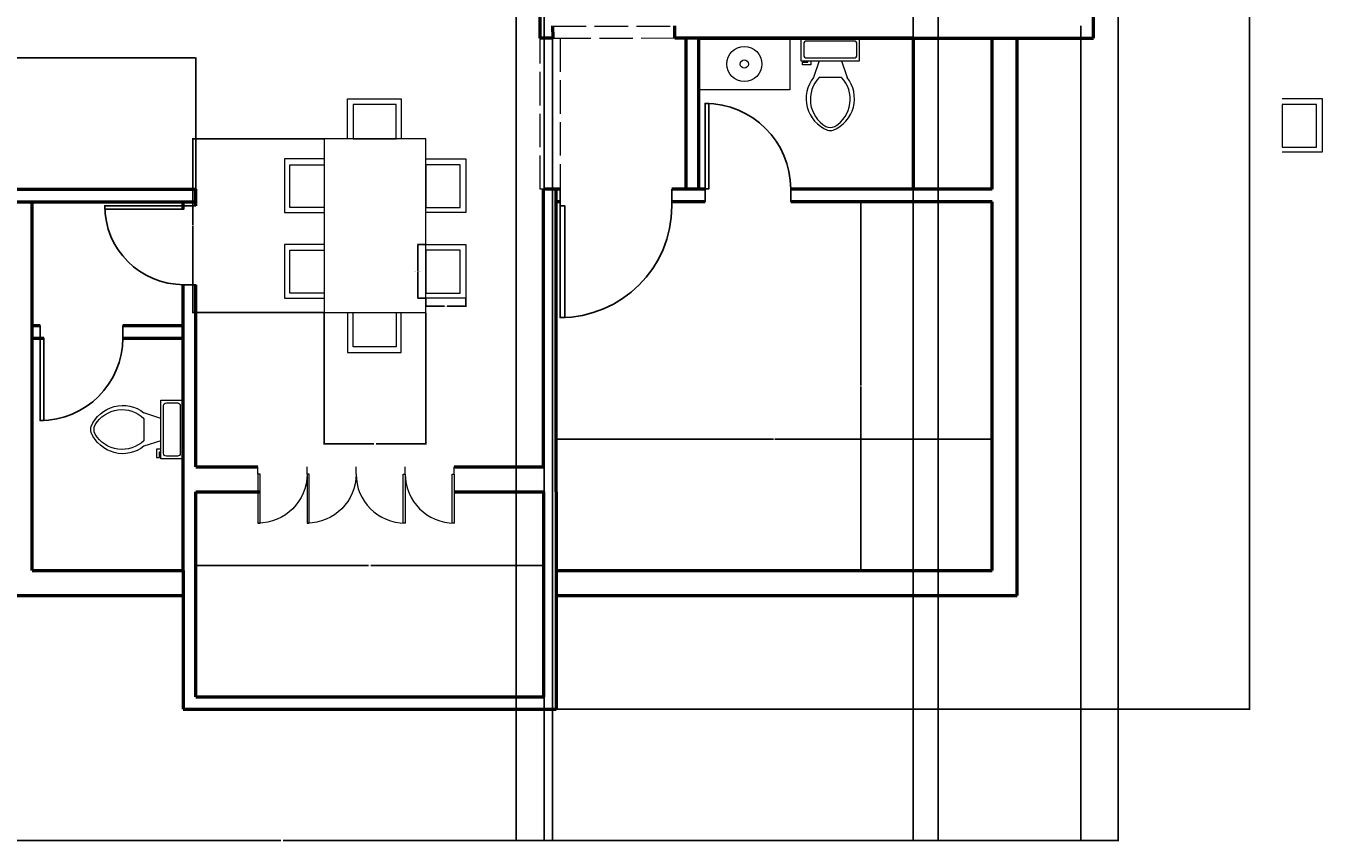
# Model space of a CAD drawing. Units: inches. Extents: x 2032 to 3981, y 840 to 2177.
# Tile 2 of 6: x 2286 to 2750, y 840 to 1132. Entities that reach past the tile are written whole.
import ezdxf

# ---------------------------------------------------------------- set-up
doc = ezdxf.new("R2010")
doc.units = ezdxf.units.IN
doc.linetypes.add('ACAD_ISO02W100', pattern=[15, 12, -3])
for name, color, linetype, lineweight in [('A-ANNO-DIMS', 2, 'Continuous', 18), ('A-DOOR', 3, 'Continuous', 25), ('A-FLOR-FIXT', 9, 'Continuous', 18), ('A-FURN', 8, 'Continuous', 18), ('A-GLAZ', 4, 'Continuous', 18), ('A-WALL', 7, 'Continuous', 50), ('A-WALL-OVHD', 8, 'ACAD_ISO02W100', 18)]:
    doc.layers.add(name, color=color, linetype=linetype, lineweight=lineweight)
doc.styles.get("Standard").update_dxf_attribs({"font": 'arial.ttf'})
doc.dimstyles.get("Standard").update_dxf_attribs({"dimtxt": 0.18, "dimasz": 0.18, "dimexe": 0.18, "dimexo": 0.0625, "dimgap": 0.09, "dimtad": 0, "dimtih": 1, "dimtoh": 1, "dimdec": 4, "dimzin": 0, "dimdsep": 46, "dimtxsty": 'Standard', "dimcen": 0.09, "dimadec": 0, "dimazin": 0, "dimtfac": 1, "dimtdec": 4, "dimtofl": 0, "dimtmove": 0, "dimatfit": 3, "dimfxl": 1, "dimtolj": 1, "dimtzin": 0, "dimarcsym": 0})

# ---------------------------------------------------------------- blocks, each defined once
blk = doc.blocks.new('*U2')
for p, q in [((0, 0), (0, -6)), ((40, 0), (40, -6))]:
    blk.add_line(p, q)
blk.add_lwpolyline([(0, 0), (0, 40), (1.75, 40), (1.75, 0)], close=True)
blk.add_arc((0, 0), 40, 0, 90)
blk = doc.blocks.new('*U4')
for p, q in [((9.5, -6), (9.5, -2)), ((-10, -8.5), (-8, -8.5)), ((-10, -9.5), (-10, -8.5)), ((-8, -8.5), (-8, -8)), ((-7, -8), (-7, -9.5)), ((-4, -8), (-6, -14)), ((4, -8), (6, -14)), ((-7, -9.5), (-10, -9.5)), ((4, -14), (-4, -14))]:
    blk.add_line(p, q)
blk.add_lwpolyline([(10.5, -8), (10.5, 0), (-10.5, 0), (-10.5, -8)], close=True)
for points in [[(-9.5, -2), (-9.5, -6)], [(8.5, -1), (-8.5, -1)], [(-8.5, -7), (8.5, -7)]]:
    blk.add_lwpolyline(points)
for centre, radius, start, end in [((-8.62, -1.88), 0.884, 81.8699, 188.1301), ((8.62, -1.88), 0.884, 351.8699, 98.1301), ((-8.62, -6.12), 0.884, 171.8699, 278.1301), ((8.62, -6.12), 0.884, 261.8699, 8.1301), ((3.52, -21.58), 12.17, 141.4691, 247.9714), ((4.2, -21.82), 11.33, 136.3677, 238.9468), ((-3.52, -21.58), 12.17, 292.0284, 38.5307), ((-4.2, -21.82), 11.33, 301.053, 43.6321), ((0, -27.88), 4, 245.7318, 294.2682), ((0, -29), 4, 254.8605, 285.1395)]:
    blk.add_arc(centre, radius, start, end)
blk = doc.blocks.new('CHAIR-DINING')
for p, q in [((0, 0), (0, 14.22)), ((0, 14.22), (19.23, 14.22)), ((19.23, 14.22), (19.23, 0))]:
    blk.add_line(p, q)
blk.add_lwpolyline([(2.09, 0), (17.42, 0), (17.42, 12.28), (2.09, 12.28)], close=True)
blk = doc.blocks.new('*D8')
at = {"layer": 'A-ANNO-DIMS', "color": 0, "lineweight": -2, "transparency": 16777216}
for p, q in [((2429.55, 1053.69), (2426.55, 1053.69)), ((2426.73, 1053.51), (2426.73, 1044.26)), ((2426.73, 1034.64), (2426.73, 1043.89)), ((2429.55, 1034.46), (2426.55, 1034.46))]:
    blk.add_line(p, q, dxfattribs=at)
at = {"layer": 'A-ANNO-DIMS', "color": 0, "lineweight": 100, "transparency": 16777216}
for points in [[(2426.7, 1053.51), (2426.76, 1053.51), (2426.73, 1053.69)], [(2426.7, 1034.64), (2426.76, 1034.64), (2426.73, 1034.46)]]:
    blk.add_solid(points, dxfattribs=at)
at = {"layer": 'Defpoints', "color": 0, "lineweight": 100, "transparency": 16777216}
for p in [(2429.61, 1053.69), (2426.73, 1034.46), (2429.61, 1034.46)]:
    blk.add_point(p, dxfattribs=at)
at = {"layer": 'A-ANNO-DIMS', "color": 0, "transparency": 16777216, "insert": (2426.73, 1044.07), "char_height": 0.18, "attachment_point": 5}
blk.add_mtext('\\A1;DINING CHAIR 19 TYP.', dxfattribs=at)
blk = doc.blocks.new('*D9')
at = {"layer": 'A-ANNO-DIMS', "color": 0, "lineweight": -2, "transparency": 16777216}
for p, q in [((2429.61, 1034.4), (2429.61, 1031.39)), ((2443.83, 1034.4), (2443.83, 1031.39)), ((2429.79, 1031.57), (2436.2, 1031.57)), ((2443.65, 1031.57), (2437.24, 1031.57))]:
    blk.add_line(p, q, dxfattribs=at)
at = {"layer": 'A-ANNO-DIMS', "color": 0, "lineweight": 100, "transparency": 16777216}
for points in [[(2429.79, 1031.6), (2429.79, 1031.54), (2429.61, 1031.57)], [(2443.65, 1031.6), (2443.65, 1031.54), (2443.83, 1031.57)]]:
    blk.add_solid(points, dxfattribs=at)
at = {"layer": 'Defpoints', "color": 0, "lineweight": 100, "transparency": 16777216}
for p in [(2429.61, 1034.46), (2443.83, 1034.46), (2443.83, 1031.57)]:
    blk.add_point(p, dxfattribs=at)
at = {"layer": 'A-ANNO-DIMS', "color": 0, "transparency": 16777216, "insert": (2436.72, 1031.57), "char_height": 0.18, "attachment_point": 5}
blk.add_mtext('\\A1;14 TYP.', dxfattribs=at)
blk = doc.blocks.new('*D14')
at = {"layer": 'A-ANNO-DIMS', "color": 0, "lineweight": -2, "transparency": 16777216}
for p, q in [((2078.89, 1518.9), (2078.89, 840.08)), ((2677.35, 1476.9), (2677.35, 840.08)), ((2079.07, 840.26), (2377.73, 840.26)), ((2677.17, 840.26), (2378.52, 840.26))]:
    blk.add_line(p, q, dxfattribs=at)
at = {"layer": 'A-ANNO-DIMS', "color": 0, "lineweight": 100, "transparency": 16777216}
for points in [[(2079.07, 840.29), (2079.07, 840.23), (2078.89, 840.26)], [(2677.17, 840.29), (2677.17, 840.23), (2677.35, 840.26)]]:
    blk.add_solid(points, dxfattribs=at)
at = {"layer": 'Defpoints', "color": 0, "lineweight": 100, "transparency": 16777216}
for p in [(2078.89, 1518.96), (2677.35, 1476.96), (2677.35, 840.26)]:
    blk.add_point(p, dxfattribs=at)
at = {"layer": 'A-ANNO-DIMS', "color": 0, "transparency": 16777216, "insert": (2378.12, 840.26), "char_height": 0.18, "attachment_point": 5}
blk.add_mtext('\\A1;598.5', dxfattribs=at)
blk = doc.blocks.new('*D15')
at = {"layer": 'A-ANNO-DIMS', "color": 0, "lineweight": -2, "transparency": 16777216}
for p, q in [((2456.69, 1820.52), (2724.53, 1820.52)), ((2724.35, 1820.34), (2724.35, 1354.07)), ((2724.35, 887.44), (2724.35, 1353.71)), ((2476.27, 887.26), (2724.53, 887.26))]:
    blk.add_line(p, q, dxfattribs=at)
at = {"layer": 'A-ANNO-DIMS', "color": 0, "lineweight": 100, "transparency": 16777216}
for points in [[(2724.32, 1820.34), (2724.38, 1820.34), (2724.35, 1820.52)], [(2724.32, 887.44), (2724.38, 887.44), (2724.35, 887.26)]]:
    blk.add_solid(points, dxfattribs=at)
at = {"layer": 'Defpoints', "color": 0, "lineweight": 100, "transparency": 16777216}
for p in [(2456.63, 1820.52), (2476.21, 887.26), (2724.35, 887.26)]:
    blk.add_point(p, dxfattribs=at)
at = {"layer": 'A-ANNO-DIMS', "color": 0, "transparency": 16777216, "insert": (2724.35, 1353.89), "char_height": 0.18, "attachment_point": 5}
blk.add_mtext('\\A1;933.3', dxfattribs=at)
blk = doc.blocks.new('*D44')
at = {"layer": 'A-ANNO-DIMS', "color": 0, "lineweight": -2, "transparency": 16777216}
for p, q in [((2164.21, 1073.52), (2164.21, 1120.64)), ((2164.39, 1120.46), (2255.43, 1120.46)), ((2347.03, 1120.46), (2255.99, 1120.46)), ((2347.21, 1073.52), (2347.21, 1120.64))]:
    blk.add_line(p, q, dxfattribs=at)
at = {"layer": 'A-ANNO-DIMS', "color": 0, "lineweight": 100, "transparency": 16777216}
for points in [[(2164.39, 1120.49), (2164.39, 1120.43), (2164.21, 1120.46)], [(2347.03, 1120.49), (2347.03, 1120.43), (2347.21, 1120.46)]]:
    blk.add_solid(points, dxfattribs=at)
at = {"layer": 'Defpoints', "color": 0, "lineweight": 100, "transparency": 16777216}
for p in [(2347.21, 1120.46), (2164.21, 1073.46), (2347.21, 1073.46)]:
    blk.add_point(p, dxfattribs=at)
at = {"layer": 'A-ANNO-DIMS', "color": 0, "transparency": 16777216, "insert": (2255.71, 1120.46), "char_height": 0.18, "attachment_point": 5}
blk.add_mtext('\\A1;183', dxfattribs=at)
blk = doc.blocks.new('*D46')
at = {"layer": 'A-ANNO-DIMS', "color": 0, "lineweight": -2, "transparency": 16777216}
for p, q in [((2347.21, 891.82), (2347.21, 938.94)), ((2347.39, 938.76), (2409.07, 938.76)), ((2471.53, 938.76), (2409.85, 938.76)), ((2471.71, 891.82), (2471.71, 938.94))]:
    blk.add_line(p, q, dxfattribs=at)
at = {"layer": 'A-ANNO-DIMS', "color": 0, "lineweight": 100, "transparency": 16777216}
for points in [[(2347.39, 938.79), (2347.39, 938.73), (2347.21, 938.76)], [(2471.53, 938.79), (2471.53, 938.73), (2471.71, 938.76)]]:
    blk.add_solid(points, dxfattribs=at)
at = {"layer": 'Defpoints', "color": 0, "lineweight": 100, "transparency": 16777216}
for p in [(2471.71, 938.76), (2347.21, 891.76), (2471.71, 891.76)]:
    blk.add_point(p, dxfattribs=at)
at = {"layer": 'A-ANNO-DIMS', "color": 0, "transparency": 16777216, "insert": (2409.46, 938.76), "char_height": 0.18, "attachment_point": 5}
blk.add_mtext('\\A1;124.5', dxfattribs=at)
blk = doc.blocks.new('*D47')
at = {"layer": 'A-ANNO-DIMS', "color": 0, "lineweight": -2, "transparency": 16777216}
for p, q in [((2476.21, 937.02), (2476.21, 984.14)), ((2476.39, 983.96), (2553.93, 983.96)), ((2632.03, 983.96), (2554.49, 983.96)), ((2632.21, 937.02), (2632.21, 984.14))]:
    blk.add_line(p, q, dxfattribs=at)
at = {"layer": 'A-ANNO-DIMS', "color": 0, "lineweight": 100, "transparency": 16777216}
for points in [[(2476.39, 983.99), (2476.39, 983.93), (2476.21, 983.96)], [(2632.03, 983.99), (2632.03, 983.93), (2632.21, 983.96)]]:
    blk.add_solid(points, dxfattribs=at)
at = {"layer": 'Defpoints', "color": 0, "lineweight": 100, "transparency": 16777216}
for p in [(2632.21, 983.96), (2476.21, 936.96), (2632.21, 936.96)]:
    blk.add_point(p, dxfattribs=at)
at = {"layer": 'A-ANNO-DIMS', "color": 0, "transparency": 16777216, "insert": (2554.21, 983.96), "char_height": 0.18, "attachment_point": 5}
blk.add_mtext('\\A1;156', dxfattribs=at)
blk = doc.blocks.new('*D48')
at = {"layer": 'A-ANNO-DIMS', "color": 0, "lineweight": -2, "transparency": 16777216}
for p, q in [((2632.15, 1068.96), (2585.03, 1068.96)), ((2585.21, 1068.78), (2585.21, 1003.14)), ((2585.21, 937.14), (2585.21, 1002.78)), ((2632.15, 936.96), (2585.03, 936.96))]:
    blk.add_line(p, q, dxfattribs=at)
at = {"layer": 'A-ANNO-DIMS', "color": 0, "lineweight": 100, "transparency": 16777216}
for points in [[(2585.18, 1068.78), (2585.24, 1068.78), (2585.21, 1068.96)], [(2585.18, 937.14), (2585.24, 937.14), (2585.21, 936.96)]]:
    blk.add_solid(points, dxfattribs=at)
at = {"layer": 'Defpoints', "color": 0, "lineweight": 100, "transparency": 16777216}
for p in [(2585.21, 1068.96), (2632.21, 1068.96), (2632.21, 936.96)]:
    blk.add_point(p, dxfattribs=at)
at = {"layer": 'A-ANNO-DIMS', "color": 0, "transparency": 16777216, "insert": (2585.21, 1002.96), "char_height": 0.18, "attachment_point": 5}
blk.add_mtext('\\A1;132', dxfattribs=at)
blk = doc.blocks.new('*D49')
at = {"layer": 'A-ANNO-DIMS', "color": 0, "lineweight": -2, "transparency": 16777216}
for p, q in [((2393.15, 1029.19), (2393.15, 982.07)), ((2429.61, 1029.19), (2429.61, 982.07)), ((2393.33, 982.25), (2410.99, 982.25)), ((2429.43, 982.25), (2411.77, 982.25))]:
    blk.add_line(p, q, dxfattribs=at)
at = {"layer": 'A-ANNO-DIMS', "color": 0, "lineweight": 100, "transparency": 16777216}
for points in [[(2393.33, 982.28), (2393.33, 982.22), (2393.15, 982.25)], [(2429.43, 982.28), (2429.43, 982.22), (2429.61, 982.25)]]:
    blk.add_solid(points, dxfattribs=at)
at = {"layer": 'Defpoints', "color": 0, "lineweight": 100, "transparency": 16777216}
for p in [(2393.15, 1029.25), (2429.61, 1029.25), (2393.15, 982.25)]:
    blk.add_point(p, dxfattribs=at)
at = {"layer": 'A-ANNO-DIMS', "color": 0, "transparency": 16777216, "insert": (2411.38, 982.25), "char_height": 0.18, "attachment_point": 5}
blk.add_mtext('\\A1;36.46', dxfattribs=at)
blk = doc.blocks.new('*D50')
at = {"layer": 'A-ANNO-DIMS', "color": 0, "lineweight": -2, "transparency": 16777216}
for p, q in [((2393.09, 1091.52), (2345.97, 1091.52)), ((2346.15, 1091.34), (2346.15, 1060.57)), ((2346.15, 1029.43), (2346.15, 1060.2)), ((2393.09, 1029.25), (2345.97, 1029.25))]:
    blk.add_line(p, q, dxfattribs=at)
at = {"layer": 'A-ANNO-DIMS', "color": 0, "lineweight": 100, "transparency": 16777216}
for points in [[(2346.12, 1091.34), (2346.18, 1091.34), (2346.15, 1091.52)], [(2346.12, 1029.43), (2346.18, 1029.43), (2346.15, 1029.25)]]:
    blk.add_solid(points, dxfattribs=at)
at = {"layer": 'Defpoints', "color": 0, "lineweight": 100, "transparency": 16777216}
for p in [(2346.15, 1091.52), (2393.15, 1091.52), (2393.15, 1029.25)]:
    blk.add_point(p, dxfattribs=at)
at = {"layer": 'A-ANNO-DIMS', "color": 0, "transparency": 16777216, "insert": (2346.15, 1060.39), "char_height": 0.18, "attachment_point": 5}
blk.add_mtext('\\A1;62.27', dxfattribs=at)
blk = doc.blocks.new('*D56')
at = {"layer": 'A-ANNO-DIMS', "color": 0, "lineweight": -2, "transparency": 16777216}
for p, q in [((2603.93, 1136.83), (2603.93, 840.08)), ((2474.93, 1131.9), (2474.93, 840.08)), ((2475.11, 840.26), (2539.15, 840.26)), ((2603.75, 840.26), (2539.72, 840.26))]:
    blk.add_line(p, q, dxfattribs=at)
at = {"layer": 'A-ANNO-DIMS', "color": 0, "lineweight": 100, "transparency": 16777216}
for points in [[(2475.11, 840.29), (2475.11, 840.23), (2474.93, 840.26)], [(2603.75, 840.29), (2603.75, 840.23), (2603.93, 840.26)]]:
    blk.add_solid(points, dxfattribs=at)
at = {"layer": 'Defpoints', "color": 0, "lineweight": 100, "transparency": 16777216}
for p in [(2603.93, 1136.9), (2474.93, 1131.96), (2603.93, 840.26)]:
    blk.add_point(p, dxfattribs=at)
at = {"layer": 'A-ANNO-DIMS', "color": 0, "transparency": 16777216, "insert": (2539.43, 840.26), "char_height": 0.18, "attachment_point": 5}
blk.add_mtext('\\A1;129', dxfattribs=at)
blk = doc.blocks.new('*D57')
at = {"layer": 'A-ANNO-DIMS', "color": 0, "lineweight": -2, "transparency": 16777216}
for p, q in [((2612.93, 1138.58), (2612.93, 840.08)), ((2663.93, 1131.9), (2663.93, 840.08)), ((2613.11, 840.26), (2638.23, 840.26)), ((2663.75, 840.26), (2638.64, 840.26))]:
    blk.add_line(p, q, dxfattribs=at)
at = {"layer": 'A-ANNO-DIMS', "color": 0, "lineweight": 100, "transparency": 16777216}
for points in [[(2613.11, 840.29), (2613.11, 840.23), (2612.93, 840.26)], [(2663.75, 840.29), (2663.75, 840.23), (2663.93, 840.26)]]:
    blk.add_solid(points, dxfattribs=at)
at = {"layer": 'Defpoints', "color": 0, "lineweight": 100, "transparency": 16777216}
for p in [(2612.93, 1138.65), (2663.93, 1131.96), (2663.93, 840.26)]:
    blk.add_point(p, dxfattribs=at)
at = {"layer": 'A-ANNO-DIMS', "color": 0, "transparency": 16777216, "insert": (2638.43, 840.26), "char_height": 0.18, "attachment_point": 5}
blk.add_mtext('\\A1;51', dxfattribs=at)
blk = doc.blocks.new('*D65')
at = {"layer": 'A-ANNO-DIMS', "color": 0, "lineweight": -2, "transparency": 16777216}
for p, q in [((2461.93, 1358.4), (2461.93, 840.08)), ((2471.93, 1358.4), (2471.93, 840.08)), ((2462.11, 840.26), (2466.72, 840.26)), ((2471.75, 840.26), (2467.14, 840.26))]:
    blk.add_line(p, q, dxfattribs=at)
at = {"layer": 'A-ANNO-DIMS', "color": 0, "lineweight": 100, "transparency": 16777216}
for points in [[(2462.11, 840.29), (2462.11, 840.23), (2461.93, 840.26)], [(2471.75, 840.29), (2471.75, 840.23), (2471.93, 840.26)]]:
    blk.add_solid(points, dxfattribs=at)
at = {"layer": 'Defpoints', "color": 0, "lineweight": 100, "transparency": 16777216}
for p in [(2461.93, 1358.46), (2471.93, 1358.46), (2471.93, 840.26)]:
    blk.add_point(p, dxfattribs=at)
at = {"layer": 'A-ANNO-DIMS', "color": 0, "transparency": 16777216, "insert": (2466.93, 840.26), "char_height": 0.18, "attachment_point": 5}
blk.add_mtext('\\A1;10', dxfattribs=at)

msp = doc.modelspace()

# ---------------------------------------------------------------- linework, layer by layer
at = {"layer": 'A-FLOR-FIXT'}
msp.add_lwpolyline([(2527.2092, 1127.4584), (2559.8471, 1127.4584), (2559.8471, 1109.0275), (2527.2092, 1109.0275)], close=True, dxfattribs=at)
for radius in [6.2897, 1.4782]:
    msp.add_circle((2543.5282, 1118.2429), radius, dxfattribs=at)
at = {"layer": 'A-FURN'}
msp.add_lwpolyline([(2393.15, 1029.2517), (2429.61, 1029.2517), (2429.61, 1091.5219), (2393.15, 1091.5219)], close=True, dxfattribs=at)
at = {"layer": 'A-WALL'}
for p, q in [((2668.4346, 1127.4584), (2668.4346, 1239.9584)), ((2470.4346, 1127.4584), (2470.4346, 1230.9584)), ((2474.9346, 1131.9584), (2475.0017, 1127.4584)), ((2518.6525, 1127.4584), (2518.6525, 1131.9584)), ((2475.0017, 1127.4584), (2470.4346, 1127.4584)), ((2475.0017, 1127.4584), (2475.0017, 1127.4584)), ((2603.9346, 1127.4584), (2518.6525, 1127.4584)), ((2522.7092, 1073.4584), (2522.7092, 1127.4584)), ((2527.2092, 1073.4584), (2527.2092, 1127.4584)), ((2527.2092, 1127.4584), (2668.4346, 1127.4584)), ((2603.9346, 1127.4584), (2603.9346, 1073.4584)), ((2632.2092, 1073.4584), (2632.2092, 1127.4584)), ((2641.2092, 1073.4584), (2641.2092, 1127.4584)), ((2164.2092, 1073.4584), (2347.2092, 1073.4584)), ((2347.2092, 1067.5396), (2347.2092, 1073.4584)), ((2471.7092, 974.088), (2471.7092, 1073.4584)), ((2477.5882, 1073.4584), (2471.7092, 1073.4584)), ((2476.2092, 965.088), (2476.2092, 1073.4584)), ((2529.4826, 1073.4584), (2517.5882, 1073.4584)), ((2529.4826, 1073.4584), (2527.2092, 1073.4584)), ((2632.2092, 1073.4584), (2560.115, 1073.4584)), ((2632.2092, 1073.4584), (2560.115, 1073.4584)), ((2641.2092, 927.9584), (2641.2092, 1073.4584)), ((2641.2092, 1068.0997), (2641.2092, 1073.4584)), ((2641.2092, 1073.4584), (2641.2092, 1073.4584)), ((2155.2092, 1068.9584), (2347.2092, 1068.9584)), ((2288.7092, 936.9584), (2288.7092, 1068.9584)), ((2342.7092, 1066.3019), (2342.7092, 1068.9584)), ((2477.5882, 1068.9584), (2476.2092, 1068.9584)), ((2529.4826, 1068.9584), (2517.5882, 1068.9584)), ((2632.2092, 1068.9584), (2560.115, 1068.9584)), ((2632.2092, 936.9584), (2632.2092, 1068.9584)), ((2342.7092, 936.9584), (2342.7092, 1039.251)), ((2347.2092, 974.088), (2347.2092, 1039.2499)), ((2288.7092, 1024.6299), (2291.5303, 1024.6299)), ((2321.1159, 1024.6299), (2342.7092, 1024.6299)), ((2471.7092, 974.088), (2471.7092, 1022.088)), ((2288.7092, 1020.1299), (2292.8247, 1020.1299)), ((2321.1158, 1020.1299), (2342.7092, 1020.1299)), ((2347.2092, 974.088), (2369.4931, 974.088)), ((2439.7363, 974.088), (2471.7092, 974.088)), ((2347.2092, 891.7551), (2347.2092, 965.088)), ((2347.2092, 965.088), (2370.2613, 965.088)), ((2439.7363, 965.088), (2471.7092, 965.088)), ((2471.7092, 965.088), (2471.7092, 936.9584)), ((2476.2092, 965.088), (2476.2092, 936.9584)), ((2288.7092, 936.9584), (2342.7092, 936.9584)), ((2342.7092, 936.9584), (2342.7092, 887.2551)), ((2471.7092, 936.9584), (2471.7092, 891.7551)), ((2476.2092, 936.9584), (2632.2092, 936.9584)), ((2476.2092, 936.9584), (2476.2092, 887.2551)), ((2155.2092, 927.9584), (2288.7092, 927.9584)), ((2288.7092, 927.9584), (2342.7092, 927.9584)), ((2476.2092, 927.9584), (2641.2092, 927.9584)), ((2347.2092, 891.7551), (2471.7092, 891.7551)), ((2342.7092, 887.2551), (2476.2092, 887.2551))]:
    msp.add_line(p, q, dxfattribs=at)
at = {"layer": 'A-WALL-OVHD'}
for points in [[(2518.6525, 1127.4584), (2474.971, 1127.4299), (2474.971, 1131.8222), (2518.6525, 1131.8507)], [(2470.4346, 1127.4584), (2477.5882, 1127.4584), (2477.5882, 1073.4584), (2470.4346, 1073.4584)]]:
    msp.add_lwpolyline(points, close=True, dxfattribs=at)

# ---------------------------------------------------------------- block references
at = {"layer": 'A-DOOR', "xscale": 0.7658094786566564, "yscale": 0.7658094786566564, "zscale": 0.7658094786566564}
msp.add_blockref('*U2', (2529.4826, 1073.5533), dxfattribs=at)
at = {"layer": 'A-DOOR', "xscale": -1, "rotation": 180}
msp.add_blockref('*U2', (2477.5882, 1067.4584), dxfattribs=at)
at = {"layer": 'A-DOOR'}
for p, xscale, yscale, zscale, rotation in [((2342.9658, 1067.5396), -0.7072431149387246, 0.7072431149387246, 0.7072431149387246, 90), ((2291.5303, 1020.192), -0.7396393782124903, 0.7396393782124903, 0.7396393782124903, 180)]:
    msp.add_blockref('*U2', p, dxfattribs=dict(at, xscale=xscale, yscale=yscale, zscale=zscale, rotation=rotation))
at = {"layer": 'A-FLOR-FIXT'}
msp.add_blockref('*U4', (2574.2876, 1127.4584), dxfattribs=at)
at = {"layer": 'A-FLOR-FIXT', "xscale": -1, "rotation": 270}
msp.add_blockref('*U4', (2342.7092, 987.4154), dxfattribs=at)
at = {"layer": 'A-FURN'}
msp.add_blockref('CHAIR-DINING', (2401.478, 1091.522), dxfattribs=at)
for p, rotation in [((2736.043, 1105.8849), 270.0000000000029), ((2429.6101, 1084.3186), 269.9999999999977), ((2429.6101, 1053.6896), 269.9999999999965)]:
    msp.add_blockref('CHAIR-DINING', p, dxfattribs=dict(at, rotation=rotation))
at = {"layer": 'A-FURN', "extrusion": (0, 0, -1), "zscale": -1}
for p, rotation in [((-2393.15, 1084.3186), 269.9999999999994), ((-2393.15, 1053.6896), 269.9999999999982), ((-2401.478, 1029.2516), 180)]:
    msp.add_blockref('CHAIR-DINING', p, dxfattribs=dict(at, rotation=rotation))
at = {"layer": 'A-GLAZ', "yscale": 0.4390204122695697, "zscale": 0.4390204122695697, "rotation": 180}
for p, xscale in [((2369.4931, 971.4538), -0.4390204122695697), ((2387.0539, 971.4538), -0.4390204122695697), ((2422.1755, 971.4538), 0.4390204122695697), ((2439.7363, 971.4538), 0.4390204122695697)]:
    msp.add_blockref('*U2', p, dxfattribs=dict(at, xscale=xscale))

# ---------------------------------------------------------------- dimensions: what is measured, and where the dimension line sits
at = {"layer": 'A-ANNO-DIMS'}
for base, p1, p2, angle, override, picture, middle in [((2724.3537, 887.2551), (2456.6278, 1820.5217), (2476.2092, 887.2551), 90, {"dimdec": 1, "dimlfac": 1, "dimrnd": 0, "dimzin": 0, "dimdsep": 46, "dimlunit": 2}, '*D15', (2724.3537, 1353.8884)), ((2346.15, 1091.5219), (2393.15, 1029.2517), (2393.15, 1091.5219), 90, {"dimdec": 2, "dimlfac": 1, "dimrnd": 0, "dimzin": 0, "dimdsep": 46, "dimlunit": 2}, '*D50', (2346.15, 1060.3868)), ((2585.2092, 1068.9584), (2632.2092, 936.9584), (2632.2092, 1068.9584), 90, {"dimdec": 0, "dimlfac": 1, "dimrnd": 0, "dimzin": 0, "dimdsep": 46, "dimlunit": 2}, '*D48', (2585.2092, 1002.9584)), ((2393.15, 982.2517), (2429.61, 1029.2517), (2393.15, 1029.2517), 180, {"dimdec": 2, "dimlfac": 1, "dimrnd": 0, "dimzin": 0, "dimdsep": 46, "dimlunit": 2}, '*D49', (2411.38, 982.2517))]:
    dim = msp.add_linear_dim(base=base, p1=p1, p2=p2, angle=angle, dimstyle='Standard', override=override, dxfattribs=at)
    dim.commit()
    dim.dimension.update_dxf_attribs({"geometry": picture, "text_midpoint": middle})
for base, p1, p2, override, picture, middle in [((2677.3537, 840.2551), (2078.8911, 1518.9584), (2677.3537, 1476.9584), {"dimdec": 1, "dimlfac": 1, "dimrnd": 0, "dimzin": 0, "dimdsep": 46, "dimlunit": 2}, '*D14', (2378.1224, 840.2551)), ((2471.9346, 840.2551), (2461.9346, 1358.4584), (2471.9346, 1358.4584), {"dimdec": 0, "dimlfac": 1, "dimrnd": 0, "dimzin": 0, "dimdsep": 46, "dimlunit": 2}, '*D65', (2466.9346, 840.2551)), ((2603.9346, 840.2551), (2474.9346, 1131.9584), (2603.9346, 1136.8961), {"dimdec": 0, "dimlfac": 1, "dimrnd": 0, "dimzin": 0, "dimdsep": 46, "dimlunit": 2}, '*D56', (2539.4346, 840.2551)), ((2663.9346, 840.2551), (2612.9346, 1138.6461), (2663.9346, 1131.9584), {"dimdec": 0, "dimlfac": 1, "dimrnd": 0, "dimzin": 0, "dimdsep": 46, "dimlunit": 2}, '*D57', (2638.4346, 840.2551)), ((2347.2092, 1120.4584), (2164.2092, 1073.4584), (2347.2092, 1073.4584), {"dimdec": 0, "dimlfac": 1, "dimrnd": 0, "dimzin": 0, "dimdsep": 46, "dimlunit": 2}, '*D44', (2255.7092, 1120.4584)), ((2632.2092, 983.9584), (2476.2092, 936.9584), (2632.2092, 936.9584), {"dimdec": 0, "dimlfac": 1, "dimrnd": 0, "dimzin": 0, "dimdsep": 46, "dimlunit": 2}, '*D47', (2554.2092, 983.9584)), ((2471.7092, 938.7551), (2347.2092, 891.7551), (2471.7092, 891.7551), {"dimdec": 1, "dimlfac": 1, "dimrnd": 0, "dimzin": 0, "dimdsep": 46, "dimlunit": 2}, '*D46', (2409.4592, 938.7551))]:
    dim = msp.add_linear_dim(base=base, p1=p1, p2=p2, dimstyle='Standard', override=override, dxfattribs=at)
    dim.commit()
    dim.dimension.update_dxf_attribs({"geometry": picture, "text_midpoint": middle})
dim = msp.add_linear_dim(base=(2426.7254, 1034.4585), p1=(2429.61, 1053.6897), p2=(2429.61, 1034.4585), angle=270, text='DINING CHAIR <> TYP.', dimstyle='Standard', override={"dimdec": 0, "dimlfac": 1, "dimrnd": 0, "dimzin": 0, "dimdsep": 46, "dimlunit": 2}, dxfattribs=at)
dim.commit()
dim.dimension.update_dxf_attribs({"geometry": '*D8', "text_midpoint": (2426.7254, 1044.0741)})
dim = msp.add_linear_dim(base=(2443.8321, 1031.5738), p1=(2429.61, 1034.4585), p2=(2443.8321, 1034.4585), text='<> TYP.', dimstyle='Standard', override={"dimdec": 0, "dimlfac": 1, "dimrnd": 0, "dimzin": 0, "dimdsep": 46, "dimlunit": 2}, dxfattribs=at)
dim.commit()
dim.dimension.update_dxf_attribs({"geometry": '*D9', "text_midpoint": (2436.7211, 1031.5738)})

doc.saveas('drawing.dxf')
